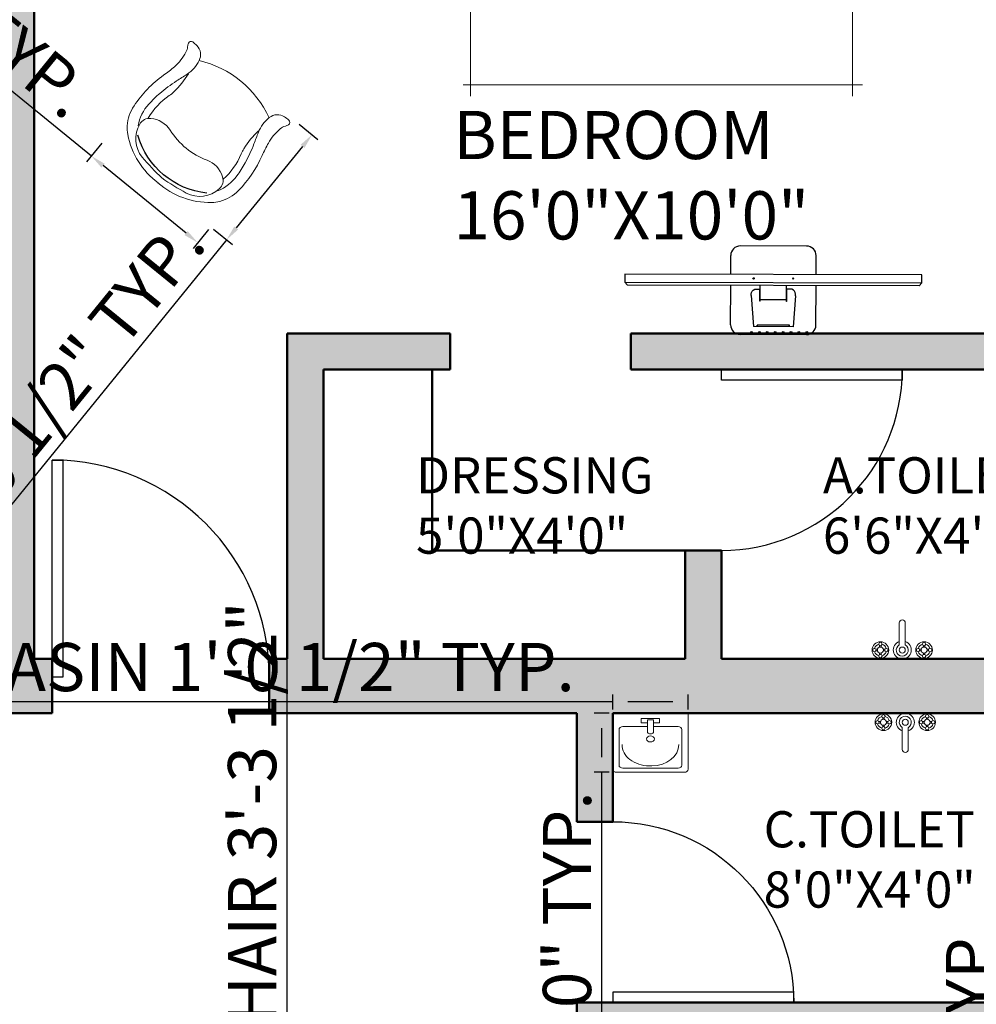
# Model space of a CAD drawing. Units: inches. Extents: x 2442 to 3851, y 589 to 2836.
# Tile 8 of 22: x 2845 to 3004, y 1717 to 1880. Entities that reach past the tile are written whole.
import ezdxf

# ---------------------------------------------------------------- set-up
doc = ezdxf.new("R2010")
doc.units = ezdxf.units.IN
for name, color, linetype, lineweight in [('0.10', 252, 'Continuous', 9), ('A-ANNO-DIMS', 2, 'Continuous', 18), ('A-AREA-IDEN', 7, 'Continuous', 18), ('A-DOOR', 4, 'Continuous', 25), ('A-FLOR-FIXT', 8, 'Continuous', 18), ('A-FURN', 8, 'Continuous', 18), ('A-WALL', 7, 'Continuous', 50), ('A-WALL-PATT', 8, 'Continuous', 13)]:
    doc.layers.add(name, color=color, linetype=linetype, lineweight=lineweight)
doc.layers.add('IFF-FURN-DETAIL', color=250, linetype='Continuous')
doc.layers.add('window', color=130, linetype='Continuous')
doc.styles.get("Standard").update_dxf_attribs({"font": 'arial.ttf'})
doc.dimstyles.new('ISO-25', dxfattribs={"dimtxt": 8, "dimasz": 2.5, "dimexe": 1.25, "dimexo": 0.625, "dimtad": 1, "dimlunit": 3, "dimtxsty": 'Standard', "dimcen": 2.5, "dimadec": 0, "dimazin": 0, "dimtfac": 1, "dimtmove": 0, "dimatfit": 3, "dimfxl": 1, "dimarcsym": 0})

# ---------------------------------------------------------------- blocks, each defined once
blk = doc.blocks.new('*U23')
for p, q in [((0, 0), (0, -6)), ((36, 0), (36, -6))]:
    blk.add_line(p, q)
blk.add_lwpolyline([(0, 0), (0, 36), (1.75, 36), (1.75, 0)], close=True)
blk.add_arc((0, 0), 36, 0, 90)
blk = doc.blocks.new('*U24')
for p, q in [((0, 0), (0, -6)), ((30, 0), (30, -6))]:
    blk.add_line(p, q)
blk.add_lwpolyline([(0, 0), (0, 30), (1.75, 30), (1.75, 0)], close=True)
blk.add_arc((0, 0), 30, 0, 90)
blk = doc.blocks.new('camita')
at = {"layer": '0.10'}
for p, q in [((-0.85, -0.045), (0.85, -0.045)), ((-0.805, -0.045), (-0.805, -2.0485)), ((0.805, -0.045), (0.805, -2.0485)), ((-0.8271, -0.521), (0.8464, -1.2932)), ((-0.8271, -0.5476), (0.8236, -1.3992)), ((-0.7161, -0.585), (-0.3554, -0.585)), ((-0.1136, -0.585), (-0.0485, -0.585)), ((-0.638, -0.63), (0.0434, -0.63)), ((0.1749, -0.63), (0.3179, -0.63)), ((0.4739, -0.63), (0.805, -0.63)), ((-0.8354, -2), (0.8464, -2))]:
    blk.add_line(p, q, dxfattribs=at)
blk.add_lwpolyline([(-0.85, -0.0405), (0.85, -0.0405), (0.85, 0), (-0.85, 0)], close=True, dxfattribs=at)
for centre, radius, start, end in [((-0.4574, -0.2364), 0.3443, 147.51, 213.8336), ((-0.1997, -0.2266), 0.5864, 163.9263, 197.1409), ((-0.3639, -5.8457), 5.7909, 83.80731, 94.12107), ((-0.5104, -1.7232), 1.6781, 80.1255, 98.6619), ((2.3534, -0.0532), 2.5803, 180.1063, 184.3854), ((-1.5443, -0.2452), 1.3333, 359.9394, 7.5533), ((1.5815, -0.2893), 1.3353, 170.3802, 178.9914), ((-1.4396, -0.0609), 1.7117, 352.9291, 0.3959), ((0.4524, -3.0675), 2.9996, 83.9026, 93.6759), ((0.4863, -1.6286), 1.5781, 80.1602, 98.06), ((0.0294, -0.1377), 0.7262, 342.5841, 6.0048), ((0.1326, -0.1696), 0.6307, 339.923, 8.7433), ((-0.0543, -0.3633), 0.4542, 159.3026, 206.5026), ((-0.007, -0.258), 0.0828, 100.018, 179.736), ((-0.2931, -1.4378), 1.2903, 61.9749, 77.8435), ((0.6265, -0.7518), 0.5508, 82.9691, 124.6739), ((0.3203, -0.3944), 0.4043, 341.4524, 33.4512), ((-1.3301, -9.6748), 9.4985, 82.27078, 84.93989), ((0.4585, -0.5454), 0.5842, 151.0456, 184.1497), ((-0.5341, -0.3393), 0.4875, 327.2644, 9.0473), ((-0.1986, -0.2742), 0.5159, 310.7395, 359.0576), ((-0.5673, -0.0868), 0.9057, 321.6953, 346.4626), ((-1.8672, -14.986), 14.6323, 84.65974, 85.75157), ((-0.4598, 1.4861), 1.9092, 260.953, 268.6517), ((0.3612, -0.133), 0.5096, 267.2589, 315.2997), ((0.4384, -0.4834), 0.1898, 193.6849, 236.7035), ((0.5707, -0.4317), 0.3145, 192.9388, 221.9636), ((-0.2002, 0.064), 0.6673, 244.7809, 279.0606), ((0.179, -0.272), 0.3828, 224.5284, 275.2229)]:
    blk.add_arc(centre, radius, start, end, dxfattribs=at)
blk = doc.blocks.new('ILNG95')
for points in [[(120, 307.8, -0.32971), (50.6, 383.9, -0.036099), (49.5, 421.7, -0.497733), (75, 439.3, -0.070621), (96.1, 428.8, 0.101868), (132.6, 413.5, 0.091794), (258.7, 412, 0.024114), (350.8, 432.5, -0.090294), (637.9, 457.7, -0.132412), (774.5, 407, -0.068618), (816.3, 367.6, -0.184346), (942.9, -0.4, 1.803905)], [(120, 307.8, 0.138132), (243.9, 312.8, 0.001085), (324.6, 339.3, -0.034227), (462.2, 374.6, -0.033255), (566.6, 386.7, -0.137428), (726.9, 350.3, -4.561553)], [(120, 307.8, 0.138132), (243.9, 312.8, 0.001085), (324.6, 339.3, -0.034227), (462.2, 374.6, -0.033255), (566.6, 386.7, -0.137428), (726.9, 350.3, -4.561553)], [(235.1, 307.5, 0.064243), (394.2, 306.7, 0.04414), (433.1, 315, -0.118032), (643, 328.5, -6.296816)], [(235.1, 307.5, 0.064243), (394.2, 306.7, 0.04414), (433.1, 315, -0.118032), (643, 328.5, -6.296816)], [(639.1, -0.4, 0.078302), (611.9, 161.3, -0.233633), (633, 315.1, -0.28763), (710.5, 349.3, -0.317923), (874.6, 193.2, -0.032882), (899.6, 0, 1.140397)], [(639.1, -0.4, 0.078302), (611.9, 161.3, -0.233633), (633, 315.1, -0.28763), (710.5, 349.3, -0.317923), (874.6, 193.2, -0.032882), (899.6, 0, 1.140397)], [(120, -307.8, 0.32971), (50.6, -383.9, 0.036099), (49.5, -421.7, 0.497733), (75, -439.3, 0.070621), (96.1, -428.8, -0.101868), (132.6, -413.5, -0.091794), (258.7, -412, -0.024114), (350.8, -432.5, 0.090294), (637.9, -457.7, 0.132412), (774.5, -407, 0.068618), (816.3, -367.6, 0.184346), (942.9, 0.4, -1.803905)], [(639.1, 0.4, -0.078302), (611.9, -161.3, 0.233633), (633, -315.1, 0.28763), (710.5, -349.3, 0.317923), (874.6, -193.2, 0.032882), (899.6, 0, -1.140397)], [(639.1, 0.4, -0.078302), (611.9, -161.3, 0.233633), (633, -315.1, 0.28763), (710.5, -349.3, 0.317923), (874.6, -193.2, 0.032882), (899.6, 0, -1.140397)], [(120, -307.8, -0.138132), (243.9, -312.8, -0.001085), (324.6, -339.3, 0.034227), (462.2, -374.6, 0.033255), (566.6, -386.7, 0.137428), (726.9, -350.3, 4.561553)], [(120, -307.8, -0.138132), (243.9, -312.8, -0.001085), (324.6, -339.3, 0.034227), (462.2, -374.6, 0.033255), (566.6, -386.7, 0.137428), (726.9, -350.3, 4.561553)], [(235.1, -307.5, -0.064243), (394.2, -306.7, -0.04414), (433.1, -315, 0.118032), (643, -328.5, 6.296816)], [(235.1, -307.5, -0.064243), (394.2, -306.7, -0.04414), (433.1, -315, 0.118032), (643, -328.5, 6.296816)]]:
    blk.add_lwpolyline(points, format="xyb")
blk.add_arc((758.7, 0.8), 708.7, 154.32815, 205.80105)
at = {"layer": 'IFF-FURN-DETAIL'}
blk.add_arc((326.4, -1.7), 549.3, 326.8997, 34.66912, dxfattribs=at)
blk.add_arc((326.4, -1.7), 549.3, 326.8997, 34.66912, dxfattribs=at)
blk = doc.blocks.new('TV')
at = {"color": 0}
for p, q in [((3967.269, 1784.848), (3967.048, 1784.654)), ((3967.765, 1763.677), (3967.535, 1763.861))]:
    blk.add_line(p, q, dxfattribs=at)
at = {"layer": 'window'}
for p, q in [((3967.535, 1763.861), (3967.048, 1784.654)), ((3964.405, 1777.232), (3967.221, 1777.298)), ((3968.009, 1777.316), (3969.36, 1777.348)), ((3966.535, 1775.819), (3964.331, 1775.605)), ((3964.337, 1775.337), (3964.45, 1775.34)), ((3964.337, 1775.315), (3964.428, 1775.317)), ((3966.143, 1775.199), (3967.01, 1775.22)), ((3966.144, 1775.177), (3966.143, 1775.199)), ((3966.144, 1775.177), (3967.27, 1775.203)), ((3966.3, 1773.288), (3966.256, 1775.179)), ((3966.188, 1773.285), (3967.314, 1773.311)), ((3966.188, 1773.262), (3966.188, 1773.285)), ((3966.188, 1773.262), (3967.055, 1773.283)), ((3964.39, 1773.063), (3964.48, 1773.065)), ((3964.391, 1773.04), (3964.503, 1773.043)), ((3966.608, 1772.662), (3964.397, 1772.772)), ((3964.548, 1771.151), (3967.363, 1771.217)), ((3968.151, 1771.235), (3969.503, 1771.267))]:
    blk.add_line(p, q, dxfattribs=at)
for points in [[(3968.328, 1763.69), (3967.832, 1784.861), (3967.269, 1784.848), (3967.765, 1763.677), (3968.328, 1763.69)], [(3970.163, 1771.958), (3970.052, 1776.688)], [(3963.856, 1771.811), (3963.745, 1776.54)], [(3964.397, 1772.772), (3964.331, 1775.605)], [(3964.48, 1773.065), (3964.428, 1775.317)], [(3964.503, 1773.043), (3964.45, 1775.34)]]:
    blk.add_lwpolyline(points, dxfattribs=at)
for points in [[(3966.535, 1775.819, -0.263666), (3966.933, 1775.689), (3967.001, 1775.572), (3967.01, 1775.22)], [(3966.608, 1772.662, 0.263666), (3967, 1772.811), (3967.063, 1772.93), (3967.055, 1773.283)]]:
    blk.add_lwpolyline(points, format="xyb", dxfattribs=at)
for centre, radius in [((3963.914, 1775.731), 0.0679), ((3967.766, 1775.678), 0.0451), ((3963.927, 1775.168), 0.0679), ((3963.94, 1774.605), 0.0679), ((3963.953, 1774.042), 0.0679), ((3963.966, 1773.478), 0.0679), ((3963.979, 1772.915), 0.0679), ((3967.832, 1772.86), 0.0451), ((3963.993, 1772.352), 0.0679), ((3964.006, 1771.789), 0.0679)]:
    blk.add_circle(centre, radius, dxfattribs=at)
for centre, start, end in [((3964.421, 1776.556), 91.34137, 181.34137), ((3969.376, 1776.672), 1.34137, 91.34137), ((3964.532, 1771.826), 181.34137, 271.34137), ((3969.487, 1771.942), 271.34137, 1.34137)]:
    blk.add_arc(centre, 0.676, start, end, dxfattribs=at)
blk = doc.blocks.new('Faucet - Bathroom top')
for p, q in [((-4.107, 0.125), (-4.375, 0.125)), ((-3.75, 0.4788), (-3.75, 0.75)), ((-3.5, 0.482), (-3.5, 0.75)), ((-3.1461, 0.125), (-2.875, 0.125)), ((3.143, 0.125), (2.875, 0.125)), ((3.5, 0.4788), (3.5, 0.75)), ((3.75, 0.482), (3.75, 0.75)), ((4.1039, 0.125), (4.375, 0.125)), ((-4.1039, -0.125), (-4.375, -0.125)), ((-3.75, -0.4821), (-3.75, -0.75)), ((-3.5, -0.4789), (-3.5, -0.75)), ((-3.143, -0.125), (-2.875, -0.125)), ((-0.5, -0.8639), (-0.5, -4.5)), ((0.5, -4.5), (0.5, -0.8631)), ((3.1461, -0.125), (2.875, -0.125)), ((3.5, -0.4821), (3.5, -0.75)), ((3.75, -0.4789), (3.75, -0.75)), ((4.107, -0.125), (4.375, -0.125))]:
    blk.add_line(p, q)
for centre, radius in [((-3.625, 0), 1.375), ((-4.625, 0), 0.2795), ((-3.625, 0), 0.5), ((-3.625, 1), 0.2795), ((-2.625, 0), 0.2795), ((0, 0), 0.5), ((3.625, 0), 1.375), ((2.625, 0), 0.2795), ((3.625, 0), 0.5), ((3.625, 1), 0.2795), ((4.625, 0), 0.2795), ((-3.625, -1), 0.2795), ((3.625, -1), 0.2795)]:
    blk.add_circle(centre, radius)
for centre, radius, start, end in [((-3.625, 0), 1, 105.2407, 164.2093), ((-3.625, 0), 1, 16.44125, 74.07887), ((0, 0), 1.5, 289.6514, 250.3603), ((0, 0), 1, 300.3431, 239.7554), ((3.625, 0), 1, 106.12, 164.0884), ((3.625, 0), 1, 16.23422, 73.90469), ((-3.625, 0), 1, 196.2342, 253.9047), ((-3.625, 0), 1, 286.12, 344.0884), ((3.625, 0), 1, 196.4413, 254.0789), ((3.625, 0), 1, 285.2407, 344.2093), ((0, -4.5), 0.5, 180, 0)]:
    blk.add_arc(centre, radius, start, end)
blk = doc.blocks.new('Rac7')
at = {"color": 0}
for p, q in [((-39473.6, -23808.4), (-38988.3, -23808.4)), ((-39500.6, -24232.1), (-39500.6, -23829.6)), ((-39456.5, -23859.1), (-39456.5, -24114.9)), ((-39032.4, -23838), (-39429.6, -23838)), ((-39221.1, -23854.9), (-39240.8, -23854.9)), ((-39005.4, -24114.9), (-39005.4, -23859.1)), ((-39005.4, -23859.1), (-39005.4, -23859.1)), ((-38961.3, -23829.6), (-38961.3, -24232.1)), ((-39252.5, -24185.9), (-39252.5, -24093.6)), ((-39209.4, -24185.9), (-39209.4, -24093.6)), ((-39429.6, -24136.1), (-39252.5, -24136.1)), ((-39297, -24164), (-39252.5, -24164)), ((-39297, -24193.5), (-39297, -24164)), ((-39209.4, -24136.1), (-39032.4, -24136.1)), ((-39209.4, -24164), (-39164.9, -24164)), ((-39164.9, -24164), (-39164.9, -24193.5)), ((-38961.3, -24232.1), (-39500.6, -24232.1)), ((-39164.9, -24193.5), (-39297, -24193.5)), ((-39252.5, -24185.9), (-39209.4, -24185.9))]:
    blk.add_line(p, q, dxfattribs=at)
at = {"color": 0, "extrusion": (0, 0, -1)}
for centre, major_axis, start_param, end_param in [((-39473.6, -23829.6), (-27, 0), 0, 1.570796), ((-38988.3, -23829.6), (-27, 0), 1.570796, 3.141593), ((-39429.6, -23859.1), (-27, 0), 0, 1.570796), ((-39240.8, -24007.4), (-194.1, 0), 0, 1.570796), ((-39221.1, -24007.4), (-194.1, 0), 1.570796, 3.141593), ((-39032.4, -23859.1), (-27, 0), 1.570796, 3.141593), ((-39231, -24104), (-25.3, 0), 0.552816, 2.588777), ((-39429.6, -24114.9), (-27, 0), -1.570796, 0), ((-39032.4, -24114.9), (-27, 0), -3.141593, -1.570796)]:
    blk.add_ellipse(centre, major_axis=major_axis, ratio=0.785714, start_param=start_param, end_param=end_param, dxfattribs=at)
blk.add_ellipse((-39231, -24048), major_axis=(-27.9, 0), ratio=0.785714, dxfattribs=at)
blk = doc.blocks.new('*D144')
at = {"layer": 'A-ANNO-DIMS', "color": 0, "lineweight": -2, "transparency": 16777216}
for p, q in [((2857.1, 1857.27), (2728.92, 1961.48)), ((2858.85, 1859.43), (2856.31, 1856.3)), ((2872.8, 1844.49), (2859.04, 1855.69)), ((2876.5, 1845.08), (2873.96, 1841.94))]:
    blk.add_line(p, q, dxfattribs=at)
at = {"layer": 'A-ANNO-DIMS', "color": 0, "transparency": 16777216}
for points in [[(2859.3, 1856.01), (2858.77, 1855.36), (2857.1, 1857.27)], [(2873.07, 1844.82), (2872.54, 1844.17), (2874.74, 1842.91)]]:
    blk.add_solid(points, dxfattribs=at)
at = {"layer": 'Defpoints', "color": 0, "transparency": 16777216}
for p in [(2859.25, 1859.91), (2857.1, 1857.27), (2876.9, 1845.56)]:
    blk.add_point(p, dxfattribs=at)
at = {"layer": 'A-ANNO-DIMS', "color": 0, "transparency": 16777216, "insert": (2795.04, 1913.86), "char_height": 8, "attachment_point": 5, "rotation": 320.8857}
blk.add_mtext('LOUNGE CHAIR 1\'-10 1/2" TYP.', dxfattribs=at)
blk = doc.blocks.new('*D145')
at = {"layer": 'A-ANNO-DIMS', "color": 0, "lineweight": -2, "transparency": 16777216}
for p, q in [((2891.54, 1862.58), (2894.67, 1860.03)), ((2892.13, 1858.88), (2881.12, 1845.35)), ((2877.38, 1845.17), (2880.51, 1842.62)), ((2879.54, 1843.41), (2831.21, 1783.96))]:
    blk.add_line(p, q, dxfattribs=at)
at = {"layer": 'A-ANNO-DIMS', "color": 0, "transparency": 16777216}
for points in [[(2891.8, 1859.15), (2892.45, 1858.62), (2893.7, 1860.82)], [(2880.8, 1845.61), (2881.45, 1845.09), (2879.54, 1843.41)]]:
    blk.add_solid(points, dxfattribs=at)
at = {"layer": 'Defpoints', "color": 0, "transparency": 16777216}
for p in [(2891.06, 1862.98), (2876.9, 1845.56), (2879.54, 1843.41)]:
    blk.add_point(p, dxfattribs=at)
at = {"layer": 'A-ANNO-DIMS', "color": 0, "transparency": 16777216, "insert": (2850.89, 1815.72), "char_height": 8, "attachment_point": 5, "rotation": 50.8857}
blk.add_mtext('1\'-10 1/2" TYP.', dxfattribs=at)
blk = doc.blocks.new('*D152')
at = {"layer": 'A-ANNO-DIMS', "color": 0, "lineweight": -2, "transparency": 16777216}
for p, q in [((2889.56, 1671.28), (2889.56, 1786.31)), ((2884.22, 1671.28), (2890.81, 1671.28)), ((2889.56, 1634.03), (2889.56, 1668.78)), ((2884.22, 1631.53), (2890.81, 1631.53))]:
    blk.add_line(p, q, dxfattribs=at)
at = {"layer": 'A-ANNO-DIMS', "color": 0, "transparency": 16777216}
for points in [[(2889.14, 1668.78), (2889.98, 1668.78), (2889.56, 1671.28)], [(2889.14, 1634.03), (2889.98, 1634.03), (2889.56, 1631.53)]]:
    blk.add_solid(points, dxfattribs=at)
at = {"layer": 'Defpoints', "color": 0, "transparency": 16777216}
for p in [(2883.6, 1671.28), (2889.56, 1671.28), (2883.6, 1631.53)]:
    blk.add_point(p, dxfattribs=at)
at = {"layer": 'A-ANNO-DIMS', "color": 0, "transparency": 16777216, "insert": (2884.79, 1730.04), "char_height": 8, "attachment_point": 5, "rotation": 90}
blk.add_mtext('SOFA CHAIR 3\'-3 1/2"', dxfattribs=at)
blk = doc.blocks.new('*D156')
at = {"layer": 'A-ANNO-DIMS', "color": 0, "lineweight": -2, "transparency": 16777216}
for p, q in [((3012.46, 1764.86), (3007.39, 1764.86)), ((3008.64, 1762.36), (3008.64, 1737.76)), ((3012.46, 1735.26), (3007.39, 1735.26)), ((3008.64, 1735.26), (3008.64, 1642.05))]:
    blk.add_line(p, q, dxfattribs=at)
at = {"layer": 'A-ANNO-DIMS', "color": 0, "transparency": 16777216}
for points in [[(3008.22, 1762.36), (3009.06, 1762.36), (3008.64, 1764.86)], [(3008.22, 1737.76), (3009.06, 1737.76), (3008.64, 1735.26)]]:
    blk.add_solid(points, dxfattribs=at)
at = {"layer": 'Defpoints', "color": 0, "transparency": 16777216}
for p in [(3013.08, 1764.86), (3008.64, 1735.26), (3013.08, 1735.26)]:
    blk.add_point(p, dxfattribs=at)
at = {"layer": 'A-ANNO-DIMS', "color": 0, "transparency": 16777216, "insert": (3003.88, 1687.4), "char_height": 8, "attachment_point": 5, "rotation": 90}
blk.add_mtext('WC 2\'-5 1/2" TYP.', dxfattribs=at)
blk = doc.blocks.new('*D158')
at = {"layer": 'A-ANNO-DIMS', "color": 0, "lineweight": -2, "transparency": 16777216}
for p, q in [((2943.6, 1765.49), (2943.6, 1767.98)), ((2956.06, 1765.49), (2956.06, 1767.98)), ((2943.6, 1766.73), (2798.84, 1766.73)), ((2953.56, 1766.73), (2946.1, 1766.73))]:
    blk.add_line(p, q, dxfattribs=at)
at = {"layer": 'A-ANNO-DIMS', "color": 0, "transparency": 16777216}
for points in [[(2946.1, 1767.15), (2946.1, 1766.32), (2943.6, 1766.73)], [(2953.56, 1767.15), (2953.56, 1766.32), (2956.06, 1766.73)]]:
    blk.add_solid(points, dxfattribs=at)
at = {"layer": 'Defpoints', "color": 0, "transparency": 16777216}
for p in [(2943.6, 1766.73), (2943.6, 1764.86), (2956.06, 1764.86)]:
    blk.add_point(p, dxfattribs=at)
at = {"layer": 'A-ANNO-DIMS', "color": 0, "transparency": 16777216, "insert": (2869.97, 1771.49), "char_height": 8, "attachment_point": 5}
blk.add_mtext('WASH BASIN 1\'-0 1/2" TYP.', dxfattribs=at)
blk = doc.blocks.new('*D159')
at = {"layer": 'A-ANNO-DIMS', "color": 0, "lineweight": -2, "transparency": 16777216}
for p, q in [((2942.97, 1764.86), (2940.48, 1764.86)), ((2941.73, 1762.36), (2941.73, 1757.57)), ((2942.97, 1755.07), (2940.48, 1755.07)), ((2941.73, 1755.07), (2941.73, 1696.34))]:
    blk.add_line(p, q, dxfattribs=at)
at = {"layer": 'A-ANNO-DIMS', "color": 0, "transparency": 16777216}
for points in [[(2941.31, 1762.36), (2942.15, 1762.36), (2941.73, 1764.86)], [(2941.31, 1757.57), (2942.15, 1757.57), (2941.73, 1755.07)]]:
    blk.add_solid(points, dxfattribs=at)
at = {"layer": 'Defpoints', "color": 0, "transparency": 16777216}
for p in [(2943.6, 1764.86), (2941.73, 1755.07), (2943.6, 1755.07)]:
    blk.add_point(p, dxfattribs=at)
at = {"layer": 'A-ANNO-DIMS', "color": 0, "transparency": 16777216, "insert": (2937.02, 1724.46), "char_height": 8, "attachment_point": 5, "rotation": 90}
blk.add_mtext('0\'-10" TYP.', dxfattribs=at)

msp = doc.modelspace()

# ---------------------------------------------------------------- hatches: boundary and pattern name
at = {"layer": 'A-WALL-PATT'}
h = msp.add_hatch(color=256, dxfattribs=at)
h.dxf.hatch_style = 1
h.paths.add_polyline_path([(2799.599, 1467.864), (2775.599, 1467.864), (2775.599, 1458.864), (2799.599, 1458.864)])
h.paths.add_polyline_path([(2703.599, 1506.864), (2670.599, 1506.864), (2670.599, 1497.864), (2694.599, 1497.864), (2694.599, 1458.864), (2733.599, 1458.864), (2733.599, 1467.864), (2709.417, 1467.864), (2703.599, 1467.864)])
h.paths.add_polyline_path([(2604.599, 1506.864), (2593.599, 1506.864), (2593.599, 1497.864), (2604.599, 1497.864)])
h.paths.add_polyline_path([(2547.599, 1497.864), (2553.599, 1497.864), (2553.599, 1506.864), (2547.599, 1506.864), (2547.599, 1530.864), (2538.599, 1530.864), (2538.599, 1401.864), (2547.599, 1401.864)])
h.paths.add_polyline_path([(2547.599, 1683.864), (2538.599, 1683.864), (2538.599, 1578.864), (2547.599, 1578.864), (2547.599, 1602.864), (2694.599, 1602.864), (2694.599, 1554.864), (2703.599, 1554.864), (2703.599, 1716.864), (2694.599, 1716.864), (2694.599, 1611.864), (2547.599, 1611.864)])
h.paths.add_polyline_path([(2892.599, 1497.864), (2883.599, 1497.864), (2883.599, 1488.228), (2883.599, 1467.864), (2865.599, 1467.864), (2865.599, 1458.864), (2892.599, 1458.864)])
h.paths.add_polyline_path([(3048.599, 1722.864), (3039.599, 1722.864), (3039.599, 1716.864), (2937.599, 1716.864), (2937.599, 1710.864), (3039.599, 1710.864), (3039.599, 1685.364), (3048.599, 1685.364)])
h.paths.add_polyline_path([(3048.599, 1779.864), (3039.599, 1779.864), (3039.599, 1773.864), (2961.599, 1773.864), (2961.599, 1791.864), (2955.599, 1791.864), (2955.599, 1773.864), (2895.599, 1773.864), (2895.599, 1821.864), (2916.599, 1821.864), (2916.599, 1827.864), (2889.599, 1827.864), (2889.599, 1773.864), (2886.599, 1773.864), (2886.599, 1764.864), (2937.599, 1764.864), (2937.599, 1746.864), (2943.599, 1746.864), (2943.599, 1764.864), (2956.06, 1764.864), (3039.599, 1764.864), (3039.599, 1758.864), (3048.599, 1758.864)])
h.paths.add_polyline_path([(3048.599, 1827.864), (2976.475, 1827.864, -0.1284593), (2975.705, 1827.665), (2964.694, 1827.687, -0.1198794), (2963.972, 1827.864), (2946.599, 1827.864), (2946.599, 1821.864), (3039.599, 1821.864), (3039.599, 1815.864), (3048.599, 1815.864)])
h.paths.add_polyline_path([(3048.599, 1956.864), (3023.366, 1956.864), (3023.277, 1956.402), (3023.088, 1956.864), (3019.494, 1956.864), (3019.543, 1955.479), (3019.146, 1956.864), (3015.599, 1956.864), (3015.599, 1947.864), (3039.599, 1947.864), (3039.599, 1875.864), (3048.599, 1875.864), (3048.599, 1880.743), (3047.576, 1881.614), (3046.081, 1883.417), (3044.931, 1885.453), (3047.541, 1883.949), (3048.599, 1883.343), (3048.599, 1910.588), (3047.049, 1909.235), (3047.896, 1910.862), (3048.599, 1911.909), (3048.599, 1918.826), (3042.477, 1917.032), (3043.928, 1918.154), (3045.59, 1919.165), (3047.525, 1920.009), (3048.599, 1920.305), (3048.599, 1926.579), (3047.576, 1927.45), (3046.081, 1929.252), (3044.931, 1931.289), (3047.541, 1929.785), (3048.599, 1929.179)])
h.paths.add_polyline_path([(2967.599, 1956.864), (2932.171, 1956.864), (2932.082, 1956.402), (2931.893, 1956.864), (2928.299, 1956.864), (2928.348, 1955.479), (2927.951, 1956.864), (2898.599, 1956.864), (2898.599, 1947.864), (2967.599, 1947.864)])
h.paths.add_polyline_path([(2850.599, 1956.864), (2834.118, 1956.864), (2834.029, 1956.402), (2833.84, 1956.864), (2830.245, 1956.864), (2830.294, 1955.479), (2829.897, 1956.864), (2796.599, 1956.864), (2796.599, 1947.864), (2799.599, 1947.864), (2838.599, 1947.864), (2838.599, 1827.864), (2835.599, 1827.864), (2835.599, 1824.864), (2835.599, 1818.864), (2838.599, 1818.864), (2838.599, 1764.864), (2850.599, 1764.864), (2850.599, 1770.864), (2850.599, 1773.864), (2847.599, 1773.864), (2847.599, 1947.864), (2850.599, 1947.864)])
h.paths.add_polyline_path([(2700.599, 1947.864), (2730.599, 1947.864), (2730.599, 1956.864), (2700.599, 1956.864), (2700.599, 1992.864), (2691.599, 1992.864), (2691.599, 1932.864), (2670.599, 1932.864), (2670.599, 1923.864), (2691.599, 1923.864), (2691.599, 1818.864), (2799.599, 1818.864), (2799.599, 1827.864), (2700.599, 1827.864)])
h.paths.add_polyline_path([(2640.599, 1932.864), (2538.599, 1932.864), (2538.599, 1868.364), (2547.599, 1868.364), (2547.599, 1923.864), (2640.599, 1923.864), (2640.599, 1929.864)])
h.paths.add_polyline_path([(2547.599, 1820.364), (2538.599, 1820.364), (2538.599, 1731.864), (2547.599, 1731.864), (2547.599, 1755.864), (2694.599, 1755.864), (2694.599, 1752.864), (2697.599, 1752.864), (2703.599, 1752.864), (2703.599, 1764.864), (2547.599, 1764.864)])
h.paths.add_polyline_path([(2725.858, 1838.187), (2790.115, 1838.187), (2790.115, 1868.602), (2725.858, 1868.602)], flags=25)
h.paths.add_polyline_path([(2892.599, 1671.864), (2883.599, 1671.864), (2883.599, 1563.864), (2892.599, 1563.864), (2892.599, 1602.864), (3048.599, 1602.864), (3048.599, 1637.364), (3039.599, 1637.364), (3039.599, 1611.864), (2892.599, 1611.864)])

# ---------------------------------------------------------------- linework, layer by layer
at = {"layer": 'A-WALL'}
for p, q in [((2847.599, 1773.864), (2847.599, 1947.864)), ((2889.599, 1827.864), (2916.599, 1827.864)), ((2889.599, 1773.864), (2889.599, 1827.864)), ((2916.599, 1821.864), (2916.599, 1827.864)), ((2946.599, 1827.864), (3048.599, 1827.864)), ((2946.599, 1821.864), (2946.599, 1827.864)), ((2895.599, 1821.864), (2916.599, 1821.864)), ((2895.599, 1773.864), (2895.599, 1821.864)), ((2913.599, 1791.864), (2913.599, 1821.864)), ((2946.599, 1821.864), (3039.599, 1821.864)), ((2913.599, 1791.864), (2955.599, 1791.864)), ((2955.599, 1773.864), (2955.599, 1791.864)), ((2955.599, 1791.864), (2961.599, 1791.864)), ((2961.599, 1773.864), (2961.599, 1791.864)), ((2847.599, 1773.864), (2850.599, 1773.864)), ((2850.599, 1764.864), (2850.599, 1773.864)), ((2886.599, 1764.864), (2886.599, 1773.864)), ((2886.599, 1773.864), (2889.599, 1773.864)), ((2895.599, 1773.864), (2955.599, 1773.864)), ((2961.599, 1773.864), (3039.599, 1773.864)), ((2838.599, 1764.864), (2850.599, 1764.864)), ((2886.599, 1764.864), (2937.599, 1764.864)), ((2937.599, 1746.864), (2937.599, 1764.864)), ((2943.599, 1764.864), (3039.599, 1764.864)), ((2943.599, 1746.864), (2943.599, 1764.864)), ((2937.599, 1746.864), (2943.599, 1746.864)), ((2937.599, 1716.864), (3039.599, 1716.864)), ((2937.599, 1710.864), (2937.599, 1716.864))]:
    msp.add_line(p, q, dxfattribs=at)

# ---------------------------------------------------------------- block references
at = {"layer": 'A-DOOR', "rotation": 269.9999999999969}
msp.add_blockref('*U24', (2961.599, 1821.864), dxfattribs=at)
at = {"layer": 'A-DOOR'}
msp.add_blockref('*U23', (2850.599, 1770.864), dxfattribs=at)
at = {"layer": 'A-DOOR', "xscale": -1, "rotation": 270}
msp.add_blockref('*U24', (2943.599, 1716.864), dxfattribs=at)
at = {"layer": 'A-FLOR-FIXT', "xscale": -1, "rotation": 180}
msp.add_blockref('Faucet - Bathroom top', (2991.598, 1775.345), dxfattribs=at)
at = {"layer": 'A-FLOR-FIXT', "xscale": 0.0231094998546128, "yscale": 0.0231094998546128, "zscale": 0.0231094998546128, "rotation": 179.9999999999958}
msp.add_blockref('Rac7', (2043.222, 1204.872), dxfattribs=at)
at = {"layer": 'A-FLOR-FIXT'}
msp.add_blockref('Faucet - Bathroom top', (2992.102, 1763.364), dxfattribs=at)
at = {"layer": 'A-FURN', "xscale": 39.375, "yscale": 39.375, "zscale": 39.375}
msp.add_blockref('camita', (2951.652, 1947.864), dxfattribs=at)
at = {"layer": 'A-FURN'}
for name, p, xscale, yscale, zscale, rotation in [('ILNG95', (2882.638, 1870.651), -0.0243705291132055, 0.0243705291132055, 0.0243705291132055, 50.88565426608293), ('TV', (6863.389, -7499.355), 2.327319231123021, 2.327319231123021, 2.327319231123021, 88.54308451816127)]:
    msp.add_blockref(name, p, dxfattribs=dict(at, xscale=xscale, yscale=yscale, zscale=zscale, rotation=rotation))

# ---------------------------------------------------------------- texts
at = {"layer": 'A-AREA-IDEN', "attachment_point": 1}
for s, insert, char_height in [('{\\fTimes New Roman|b0|i0|c0|p18;BEDROOM\\P16\'0"X10\'0"}', (2917.154, 1864.776), 8), ('{\\fTimes New Roman|b0|i0|c0|p18;DRESSING\\P5\'0"X4\'0"}', (2910.952, 1807.325), 6), ('{\\fTimes New Roman|b0|i0|c0|p18;A.TOILET\\P6\'6"X4\'0"}', (2978.437, 1807.325), 6), ('{\\fTimes New Roman|b0|i0|c0|p18;C.TOILET\\P8\'0"X4\'0"}', (2968.612, 1748.618), 6)]:
    msp.add_mtext_dynamic_manual_height_columns(s, width=110.76054, gutter_width=12.5, heights=[0], dxfattribs=dict(at, insert=insert, char_height=char_height))

# ---------------------------------------------------------------- dimensions: what is measured, and where the dimension line sits
at = {"layer": 'A-ANNO-DIMS'}
for base, p1, p2, angle, text, picture, middle in [((2857.095, 1857.265), (2876.897, 1845.562), (2859.248, 1859.913), 140.88565, 'LOUNGE CHAIR <> TYP.', '*D144', (2795.044, 1913.859)), ((2879.545, 1843.409), (2891.056, 1862.976), (2876.897, 1845.562), 230.88565, '<> TYP.', '*D145', (2850.894, 1815.72)), ((2943.599, 1766.733), (2956.06, 1764.864), (2943.599, 1764.864), 180, 'WASH BASIN <> TYP.', '*D158', (2869.969, 1771.495)), ((2889.56, 1671.277), (2883.599, 1631.534), (2883.599, 1671.277), 90, 'SOFA CHAIR <>', '*D152', (2884.793, 1730.042)), ((2941.729, 1755.073), (2943.599, 1764.864), (2943.599, 1755.073), 270, '<> TYP.', '*D159', (2937.02, 1724.458)), ((3008.641, 1735.257), (3013.083, 1764.864), (3013.083, 1735.257), 270, 'WC <> TYP.', '*D156', (3003.88, 1687.403))]:
    dim = msp.add_linear_dim(base=base, p1=p1, p2=p2, angle=angle, text=text, dimstyle='ISO-25', override={"dimdec": 1, "dimrnd": 0, "dimzin": 1, "dimlunit": 4, "dimfrac": 2}, dxfattribs=at)
    dim.commit()
    dim.dimension.update_dxf_attribs({"geometry": picture, "text_midpoint": middle})

doc.saveas('drawing.dxf')
